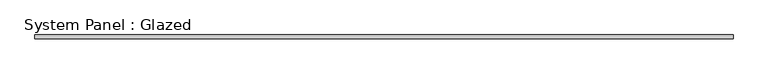
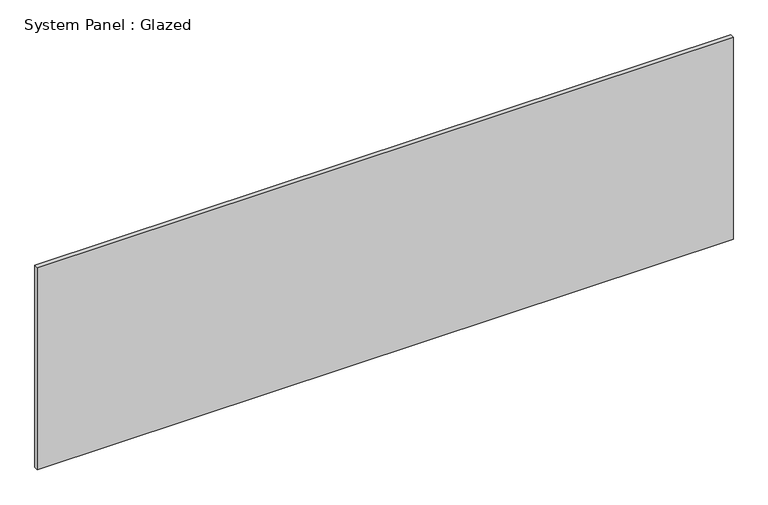
"""IFC4 building model written with IfcOpenShell, lengths in millimetres: plate geometry, System Panel : Glazed."""

from ifc_helpers import new_model, si_unit, origin, origin_with_axes, place, context, project, spatial, polyline, outline, extrude, source, transform, mapped, element, save


def system_panel_glazed_6b509a71(model_context):
    return source(origin(), model_context, "Body", "SweptSolid", [
        extrude(outline(polyline([(2378.9332138, 19.05), (-2378.9332138, 19.05), (-2378.9332138, 44.45), (2378.9332138, 44.45), (2378.9332138, 19.05)])), origin_with_axes(), (0.0, 0.0, 1.0), 1460.5),
    ])


if __name__ == "__main__":
    model = new_model("IFC4")
    model_context = context("Model", 3, world=origin())
    ifc_project = project(units=[si_unit("LENGTHUNIT", "METRE", prefix="MILLI")], contexts=[model_context])
    site = spatial("IfcSite", under=ifc_project)
    building = spatial("IfcBuilding", under=site)
    placement = place(None, origin())
    system_panel_glazed_shape = system_panel_glazed_6b509a71(model_context)
    element("IfcPlate", 1, ObjectType="System Panel : Glazed", at=placement, inside=building, context=model_context, shape_type="MappedRepresentation", body=[
        mapped(system_panel_glazed_shape, transform((0.0, 0.0, 0.0), x_axis=(1.0, 0.0, 0.0), y_axis=(0.0, 1.0, 0.0), z_axis=(0.0, 0.0, 1.0))),
    ])
    save(model, "model.ifc")

# Revit data of these elements
# Type "System Panel : Glazed"
#   Construction Type Id = "GSP4R"
#   Analytic Construction = "1/8 in Pilkington single glazing"
#   Visual Light Transmittance = 0.9
#   Solar Heat Gain Coefficient = 0.86
#   Heat Transfer Coefficient (U) = 1.18115 BTU/(h·ft²·°F)
# Element 1 (IfcPlate, "System Panel : Glazed")
#   Materials on its faces: "Glass"
# Materials
#   "Glass": class "Glass", colour RGB 0 128 192, transparency 0.75, Description = "Soda Lime Glass", Cost = 0
